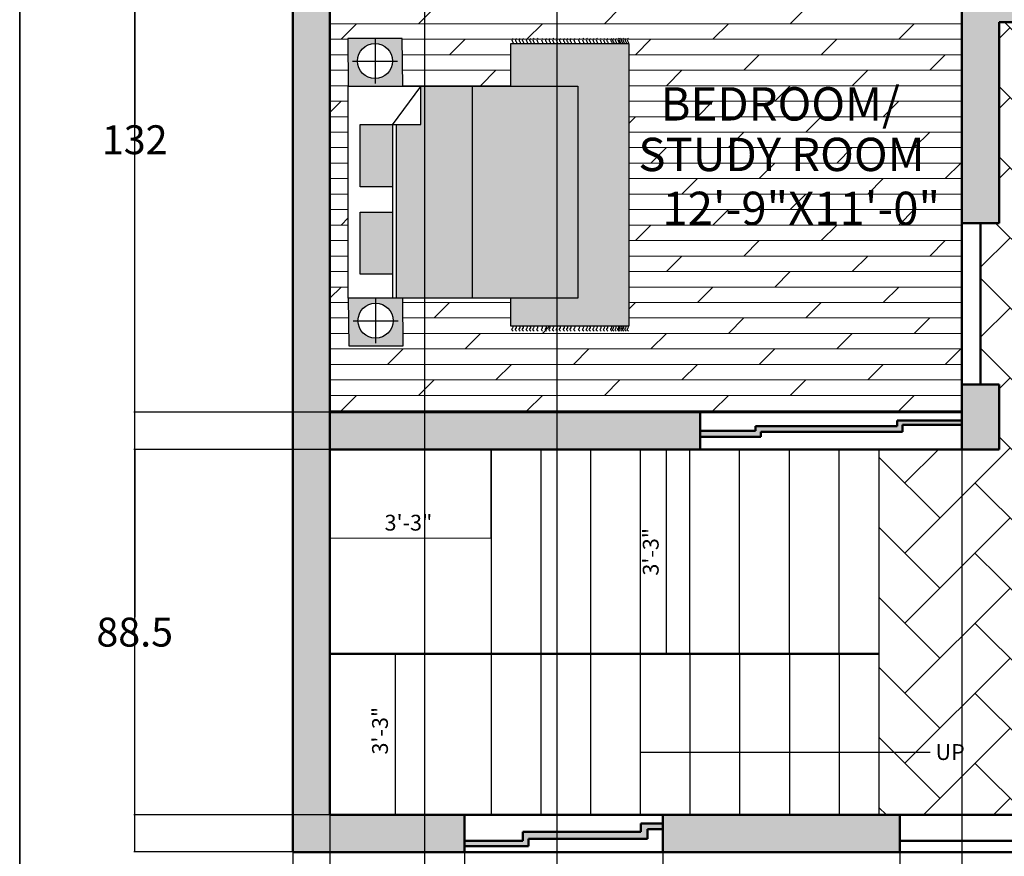
# Model space of a CAD drawing. Units: inches. Extents: x 1381 to 2246, y 1317 to 2168.
# Tile 2 of 15: x 1381 to 1619, y 1471 to 1673. Entities that reach past the tile are written whole.
import ezdxf

# ---------------------------------------------------------------- set-up
doc = ezdxf.new("R2010")
doc.units = ezdxf.units.IN
doc.header["$MEASUREMENT"] = 0
for name, color, linetype, lineweight in [('A-ANNO-DIMS', 2, 'Continuous', 18), ('A-ANNO-TEXT', 7, 'Continuous', 18), ('A-ANNO-TTLB', 7, 'Continuous', 35), ('A-AREA-IDEN', 3, 'Continuous', 25), ('A-FLOR-PATT', 252, 'Continuous', 13), ('A-FLOR-STRS', 3, 'Continuous', 25), ('A-FURN', 8, 'Continuous', 18), ('A-GLAZ', 4, 'Continuous', 25), ('A-WALL', 7, 'Continuous', 50)]:
    doc.layers.add(name, color=color, linetype=linetype, lineweight=lineweight)
doc.layers.add('furniture', color=250, linetype='Continuous')
doc.styles.get("Standard").update_dxf_attribs({"font": 'arial.ttf'})
doc.dimstyles.get("Standard").update_dxf_attribs({"dimtxt": 7, "dimasz": 0.18, "dimexe": 0.18, "dimexo": 0.0625, "dimgap": 0.09, "dimtad": 0, "dimtih": 1, "dimtoh": 1, "dimdec": 1, "dimzin": 0, "dimdsep": 46, "dimlunit": 3, "dimtxsty": 'Standard', "dimcen": 0.09, "dimadec": 0, "dimazin": 0, "dimtfac": 1, "dimtdec": 1, "dimtofl": 0, "dimtmove": 0, "dimatfit": 3, "dimfxl": 1, "dimtolj": 1, "dimtzin": 0, "dimarcsym": 0})

# ---------------------------------------------------------------- blocks, each defined once
blk = doc.blocks.new('CARPET')
at = {"layer": 'furniture'}
for p, q in [((-51.53, -98.11), (-51.53, -55.12)), ((-51.53, -55.12), (-41.27, -55.12)), ((36, -55.12), (51.55, -55.12)), ((51.55, -55.12), (51.55, -98.11)), ((51.55, -98.11), (-51.53, -98.11))]:
    blk.add_line(p, q, dxfattribs=at)
for points, knots in [([(-53.37, -55.99), (-53.22, -55.8), (-52.9, -55.41), (-52.34, -55.8), (-51.89, -56.08), (-51.65, -55.91), (-51.53, -55.83)], [0, 0, 0, 0, 0.653278, 1.290138, 1.740457, 2.114451, 2.114451, 2.114451, 2.114451]), ([(-53.37, -57.26), (-53.22, -57.07), (-52.9, -56.67), (-52.34, -57.07), (-51.89, -57.35), (-51.65, -57.17), (-51.53, -57.1)], [0, 0, 0, 0, 0.653278, 1.290138, 1.740457, 2.114451, 2.114451, 2.114451, 2.114451]), ([(53.37, -55.99), (53.22, -55.8), (52.9, -55.41), (52.34, -55.8), (51.89, -56.08), (51.65, -55.91), (51.53, -55.83)], [0, 0, 0, 0, 0.653278, 1.290138, 1.740457, 2.114451, 2.114451, 2.114451, 2.114451]), ([(53.37, -57.26), (53.22, -57.07), (52.9, -56.67), (52.34, -57.07), (51.89, -57.35), (51.65, -57.17), (51.53, -57.1)], [0, 0, 0, 0, 0.653278, 1.290138, 1.740457, 2.114451, 2.114451, 2.114451, 2.114451]), ([(-53.37, -58.59), (-53.22, -58.4), (-52.9, -58.01), (-52.34, -58.4), (-51.89, -58.68), (-51.65, -58.5), (-51.53, -58.43)], [0, 0, 0, 0, 0.653278, 1.290138, 1.740457, 2.114451, 2.114451, 2.114451, 2.114451]), ([(-53.37, -59.78), (-53.22, -59.58), (-52.9, -59.19), (-52.34, -59.58), (-51.89, -59.86), (-51.65, -59.69), (-51.53, -59.61)], [0, 0, 0, 0, 0.653278, 1.290138, 1.740457, 2.114451, 2.114451, 2.114451, 2.114451]), ([(-53.37, -61.22), (-53.22, -61.02), (-52.9, -60.63), (-52.34, -61.02), (-51.89, -61.3), (-51.65, -61.13), (-51.53, -61.05)], [0, 0, 0, 0, 0.653278, 1.290138, 1.740457, 2.114451, 2.114451, 2.114451, 2.114451]), ([(53.37, -58.59), (53.22, -58.4), (52.9, -58.01), (52.34, -58.4), (51.89, -58.68), (51.65, -58.5), (51.53, -58.43)], [0, 0, 0, 0, 0.653278, 1.290138, 1.740457, 2.114451, 2.114451, 2.114451, 2.114451]), ([(53.37, -59.78), (53.22, -59.58), (52.9, -59.19), (52.34, -59.58), (51.89, -59.86), (51.65, -59.69), (51.53, -59.61)], [0, 0, 0, 0, 0.653278, 1.290138, 1.740457, 2.114451, 2.114451, 2.114451, 2.114451]), ([(53.37, -61.22), (53.22, -61.02), (52.9, -60.63), (52.34, -61.02), (51.89, -61.3), (51.65, -61.13), (51.53, -61.05)], [0, 0, 0, 0, 0.653278, 1.290138, 1.740457, 2.114451, 2.114451, 2.114451, 2.114451]), ([(-53.37, -62.44), (-53.22, -62.25), (-52.9, -61.86), (-52.34, -62.25), (-51.89, -62.53), (-51.65, -62.36), (-51.53, -62.28)], [0, 0, 0, 0, 0.653278, 1.290138, 1.740457, 2.114451, 2.114451, 2.114451, 2.114451]), ([(-53.37, -63.63), (-53.22, -63.43), (-52.9, -63.04), (-52.34, -63.43), (-51.89, -63.72), (-51.65, -63.54), (-51.53, -63.46)], [0, 0, 0, 0, 0.653278, 1.290138, 1.740457, 2.114451, 2.114451, 2.114451, 2.114451]), ([(53.37, -62.44), (53.22, -62.25), (52.9, -61.86), (52.34, -62.25), (51.89, -62.53), (51.65, -62.36), (51.53, -62.28)], [0, 0, 0, 0, 0.653278, 1.290138, 1.740457, 2.114451, 2.114451, 2.114451, 2.114451]), ([(53.37, -63.63), (53.22, -63.43), (52.9, -63.04), (52.34, -63.43), (51.89, -63.72), (51.65, -63.54), (51.53, -63.46)], [0, 0, 0, 0, 0.653278, 1.290138, 1.740457, 2.114451, 2.114451, 2.114451, 2.114451]), ([(-53.37, -65.07), (-53.22, -64.87), (-52.9, -64.48), (-52.34, -64.87), (-51.89, -65.15), (-51.65, -64.98), (-51.53, -64.9)], [0, 0, 0, 0, 0.653278, 1.290138, 1.740457, 2.114451, 2.114451, 2.114451, 2.114451]), ([(-53.37, -66.76), (-53.22, -66.56), (-52.9, -66.17), (-52.34, -66.56), (-51.89, -66.84), (-51.65, -66.67), (-51.53, -66.59)], [0, 0, 0, 0, 0.653278, 1.290138, 1.740457, 2.114451, 2.114451, 2.114451, 2.114451]), ([(-53.37, -68.2), (-53.22, -68), (-52.9, -67.61), (-52.34, -68), (-51.89, -68.28), (-51.65, -68.11), (-51.53, -68.03)], [0, 0, 0, 0, 0.653278, 1.290138, 1.740457, 2.114451, 2.114451, 2.114451, 2.114451]), ([(53.37, -65.07), (53.22, -64.87), (52.9, -64.48), (52.34, -64.87), (51.89, -65.15), (51.65, -64.98), (51.53, -64.9)], [0, 0, 0, 0, 0.653278, 1.290138, 1.740457, 2.114451, 2.114451, 2.114451, 2.114451]), ([(53.37, -66.76), (53.22, -66.56), (52.9, -66.17), (52.34, -66.56), (51.89, -66.84), (51.65, -66.67), (51.53, -66.59)], [0, 0, 0, 0, 0.653278, 1.290138, 1.740457, 2.114451, 2.114451, 2.114451, 2.114451]), ([(53.37, -68.2), (53.22, -68), (52.9, -67.61), (52.34, -68), (51.89, -68.28), (51.65, -68.11), (51.53, -68.03)], [0, 0, 0, 0, 0.653278, 1.290138, 1.740457, 2.114451, 2.114451, 2.114451, 2.114451]), ([(-53.37, -69.53), (-53.22, -69.33), (-52.9, -68.94), (-52.34, -69.33), (-51.89, -69.61), (-51.65, -69.44), (-51.53, -69.36)], [0, 0, 0, 0, 0.653278, 1.290138, 1.740457, 2.114451, 2.114451, 2.114451, 2.114451]), ([(-53.37, -70.79), (-53.22, -70.6), (-52.9, -70.21), (-52.34, -70.6), (-51.89, -70.88), (-51.65, -70.7), (-51.53, -70.63)], [0, 0, 0, 0, 0.653278, 1.290138, 1.740457, 2.114451, 2.114451, 2.114451, 2.114451]), ([(-53.37, -72.12), (-53.22, -71.93), (-52.9, -71.54), (-52.34, -71.93), (-51.89, -72.21), (-51.65, -72.04), (-51.53, -71.96)], [0, 0, 0, 0, 0.653278, 1.290138, 1.740457, 2.114451, 2.114451, 2.114451, 2.114451]), ([(53.37, -69.53), (53.22, -69.33), (52.9, -68.94), (52.34, -69.33), (51.89, -69.61), (51.65, -69.44), (51.53, -69.36)], [0, 0, 0, 0, 0.653278, 1.290138, 1.740457, 2.114451, 2.114451, 2.114451, 2.114451]), ([(53.37, -70.79), (53.22, -70.6), (52.9, -70.21), (52.34, -70.6), (51.89, -70.88), (51.65, -70.7), (51.53, -70.63)], [0, 0, 0, 0, 0.653278, 1.290138, 1.740457, 2.114451, 2.114451, 2.114451, 2.114451]), ([(53.37, -72.12), (53.22, -71.93), (52.9, -71.54), (52.34, -71.93), (51.89, -72.21), (51.65, -72.04), (51.53, -71.96)], [0, 0, 0, 0, 0.653278, 1.290138, 1.740457, 2.114451, 2.114451, 2.114451, 2.114451]), ([(-53.37, -73.31), (-53.22, -73.11), (-52.9, -72.72), (-52.34, -73.11), (-51.89, -73.4), (-51.65, -73.22), (-51.53, -73.14)], [0, 0, 0, 0, 0.653278, 1.290138, 1.740457, 2.114451, 2.114451, 2.114451, 2.114451]), ([(-53.37, -74.75), (-53.22, -74.55), (-52.9, -74.16), (-52.34, -74.55), (-51.89, -74.83), (-51.65, -74.66), (-51.53, -74.58)], [0, 0, 0, 0, 0.653278, 1.290138, 1.740457, 2.114451, 2.114451, 2.114451, 2.114451]), ([(53.37, -73.31), (53.22, -73.11), (52.9, -72.72), (52.34, -73.11), (51.89, -73.4), (51.65, -73.22), (51.53, -73.14)], [0, 0, 0, 0, 0.653278, 1.290138, 1.740457, 2.114451, 2.114451, 2.114451, 2.114451]), ([(53.37, -74.75), (53.22, -74.55), (52.9, -74.16), (52.34, -74.55), (51.89, -74.83), (51.65, -74.66), (51.53, -74.58)], [0, 0, 0, 0, 0.653278, 1.290138, 1.740457, 2.114451, 2.114451, 2.114451, 2.114451]), ([(-53.37, -75.98), (-53.22, -75.78), (-52.9, -75.39), (-52.34, -75.78), (-51.89, -76.06), (-51.65, -75.89), (-51.53, -75.81)], [0, 0, 0, 0, 0.653278, 1.290138, 1.740457, 2.114451, 2.114451, 2.114451, 2.114451]), ([(-53.37, -77.16), (-53.22, -76.96), (-52.9, -76.57), (-52.34, -76.96), (-51.89, -77.25), (-51.65, -77.07), (-51.53, -76.99)], [0, 0, 0, 0, 0.653278, 1.290138, 1.740457, 2.114451, 2.114451, 2.114451, 2.114451]), ([(-53.37, -78.6), (-53.22, -78.4), (-52.9, -78.01), (-52.34, -78.4), (-51.89, -78.68), (-51.65, -78.51), (-51.53, -78.43)], [0, 0, 0, 0, 0.653278, 1.290138, 1.740457, 2.114451, 2.114451, 2.114451, 2.114451]), ([(53.37, -75.98), (53.22, -75.78), (52.9, -75.39), (52.34, -75.78), (51.89, -76.06), (51.65, -75.89), (51.53, -75.81)], [0, 0, 0, 0, 0.653278, 1.290138, 1.740457, 2.114451, 2.114451, 2.114451, 2.114451]), ([(53.37, -77.16), (53.22, -76.96), (52.9, -76.57), (52.34, -76.96), (51.89, -77.25), (51.65, -77.07), (51.53, -76.99)], [0, 0, 0, 0, 0.653278, 1.290138, 1.740457, 2.114451, 2.114451, 2.114451, 2.114451]), ([(53.37, -78.6), (53.22, -78.4), (52.9, -78.01), (52.34, -78.4), (51.89, -78.68), (51.65, -78.51), (51.53, -78.43)], [0, 0, 0, 0, 0.653278, 1.290138, 1.740457, 2.114451, 2.114451, 2.114451, 2.114451]), ([(-53.37, -80.29), (-53.22, -80.09), (-52.9, -79.7), (-52.34, -80.09), (-51.89, -80.37), (-51.65, -80.2), (-51.53, -80.12)], [0, 0, 0, 0, 0.653278, 1.290138, 1.740457, 2.114451, 2.114451, 2.114451, 2.114451]), ([(-53.37, -81.73), (-53.22, -81.53), (-52.9, -81.14), (-52.34, -81.53), (-51.89, -81.81), (-51.65, -81.64), (-51.53, -81.56)], [0, 0, 0, 0, 0.653278, 1.290138, 1.740457, 2.114451, 2.114451, 2.114451, 2.114451]), ([(53.37, -80.29), (53.22, -80.09), (52.9, -79.7), (52.34, -80.09), (51.89, -80.37), (51.65, -80.2), (51.53, -80.12)], [0, 0, 0, 0, 0.653278, 1.290138, 1.740457, 2.114451, 2.114451, 2.114451, 2.114451]), ([(53.37, -81.73), (53.22, -81.53), (52.9, -81.14), (52.34, -81.53), (51.89, -81.81), (51.65, -81.64), (51.53, -81.56)], [0, 0, 0, 0, 0.653278, 1.290138, 1.740457, 2.114451, 2.114451, 2.114451, 2.114451]), ([(-53.37, -83.06), (-53.22, -82.86), (-52.9, -82.47), (-52.34, -82.86), (-51.89, -83.14), (-51.65, -82.97), (-51.53, -82.89)], [0, 0, 0, 0, 0.653278, 1.290138, 1.740457, 2.114451, 2.114451, 2.114451, 2.114451]), ([(-53.37, -84.18), (-53.22, -83.99), (-52.9, -83.6), (-52.34, -83.99), (-51.89, -84.27), (-51.65, -84.09), (-51.53, -84.02)], [0, 0, 0, 0, 0.653278, 1.290138, 1.740457, 2.114451, 2.114451, 2.114451, 2.114451]), ([(-53.37, -85.51), (-53.22, -85.32), (-52.9, -84.93), (-52.34, -85.32), (-51.89, -85.6), (-51.65, -85.42), (-51.53, -85.35)], [0, 0, 0, 0, 0.653278, 1.290138, 1.740457, 2.114451, 2.114451, 2.114451, 2.114451]), ([(53.37, -83.06), (53.22, -82.86), (52.9, -82.47), (52.34, -82.86), (51.89, -83.14), (51.65, -82.97), (51.53, -82.89)], [0, 0, 0, 0, 0.653278, 1.290138, 1.740457, 2.114451, 2.114451, 2.114451, 2.114451]), ([(53.37, -84.18), (53.22, -83.99), (52.9, -83.6), (52.34, -83.99), (51.89, -84.27), (51.65, -84.09), (51.53, -84.02)], [0, 0, 0, 0, 0.653278, 1.290138, 1.740457, 2.114451, 2.114451, 2.114451, 2.114451]), ([(53.37, -85.51), (53.22, -85.32), (52.9, -84.93), (52.34, -85.32), (51.89, -85.6), (51.65, -85.42), (51.53, -85.35)], [0, 0, 0, 0, 0.653278, 1.290138, 1.740457, 2.114451, 2.114451, 2.114451, 2.114451]), ([(-53.37, -86.7), (-53.22, -86.5), (-52.9, -86.11), (-52.34, -86.5), (-51.89, -86.78), (-51.65, -86.61), (-51.53, -86.53)], [0, 0, 0, 0, 0.653278, 1.290138, 1.740457, 2.114451, 2.114451, 2.114451, 2.114451]), ([(-53.37, -88.14), (-53.22, -87.94), (-52.9, -87.55), (-52.34, -87.94), (-51.89, -88.22), (-51.65, -88.05), (-51.53, -87.97)], [0, 0, 0, 0, 0.653278, 1.290138, 1.740457, 2.114451, 2.114451, 2.114451, 2.114451]), ([(-53.37, -89.36), (-53.22, -89.17), (-52.9, -88.78), (-52.34, -89.17), (-51.89, -89.45), (-51.65, -89.28), (-51.53, -89.2)], [0, 0, 0, 0, 0.653278, 1.290138, 1.740457, 2.114451, 2.114451, 2.114451, 2.114451]), ([(53.37, -86.7), (53.22, -86.5), (52.9, -86.11), (52.34, -86.5), (51.89, -86.78), (51.65, -86.61), (51.53, -86.53)], [0, 0, 0, 0, 0.653278, 1.290138, 1.740457, 2.114451, 2.114451, 2.114451, 2.114451]), ([(53.37, -88.14), (53.22, -87.94), (52.9, -87.55), (52.34, -87.94), (51.89, -88.22), (51.65, -88.05), (51.53, -87.97)], [0, 0, 0, 0, 0.653278, 1.290138, 1.740457, 2.114451, 2.114451, 2.114451, 2.114451]), ([(53.37, -89.36), (53.22, -89.17), (52.9, -88.78), (52.34, -89.17), (51.89, -89.45), (51.65, -89.28), (51.53, -89.2)], [0, 0, 0, 0, 0.653278, 1.290138, 1.740457, 2.114451, 2.114451, 2.114451, 2.114451]), ([(-53.37, -90.55), (-53.22, -90.35), (-52.9, -89.96), (-52.34, -90.35), (-51.89, -90.64), (-51.65, -90.46), (-51.53, -90.38)], [0, 0, 0, 0, 0.653278, 1.290138, 1.740457, 2.114451, 2.114451, 2.114451, 2.114451]), ([(-53.37, -91.99), (-53.22, -91.79), (-52.9, -91.4), (-52.34, -91.79), (-51.89, -92.07), (-51.65, -91.9), (-51.53, -91.82)], [0, 0, 0, 0, 0.653278, 1.290138, 1.740457, 2.114451, 2.114451, 2.114451, 2.114451]), ([(-53.37, -92.69), (-53.22, -92.48), (-52.9, -92.08), (-52.35, -92.49), (-51.89, -92.77), (-51.65, -92.6), (-51.53, -92.52)], [0, 0, 0, 0, 0.663904, 1.307406, 1.757725, 2.131719, 2.131719, 2.131719, 2.131719]), ([(-53.37, -93.61), (-53.22, -93.42), (-52.9, -93.03), (-52.34, -93.42), (-51.89, -93.7), (-51.65, -93.52), (-51.53, -93.45)], [0, 0, 0, 0, 0.653278, 1.290138, 1.740457, 2.114451, 2.114451, 2.114451, 2.114451]), ([(53.37, -90.55), (53.22, -90.35), (52.9, -89.96), (52.34, -90.35), (51.9, -90.63), (51.66, -90.47), (51.55, -90.4)], [0, 0, 0, 0, 0.653278, 1.290138, 1.740457, 2.0926, 2.0926, 2.0926, 2.0926]), ([(53.37, -91.99), (53.22, -91.79), (52.9, -91.4), (52.34, -91.79), (51.9, -92.07), (51.66, -91.91), (51.55, -91.83)], [0, 0, 0, 0, 0.653278, 1.290138, 1.740457, 2.0926, 2.0926, 2.0926, 2.0926]), ([(53.37, -92.69), (53.22, -92.49), (52.9, -92.09), (52.34, -92.49), (51.9, -92.77), (51.66, -92.61), (51.55, -92.53)], [0, 0, 0, 0, 0.656792, 1.295826, 1.746145, 2.098292, 2.098292, 2.098292, 2.098292]), ([(53.37, -93.66), (53.22, -93.46), (52.9, -93.07), (52.34, -93.46), (51.9, -93.74), (51.66, -93.58), (51.55, -93.5)], [0, 0, 0, 0, 0.653278, 1.290138, 1.740457, 2.0926, 2.0926, 2.0926, 2.0926]), ([(-53.37, -94.55), (-53.22, -94.35), (-52.9, -93.96), (-52.34, -94.35), (-51.89, -94.63), (-51.65, -94.46), (-51.53, -94.38)], [0, 0, 0, 0, 0.653278, 1.290138, 1.740457, 2.114451, 2.114451, 2.114451, 2.114451]), ([(-53.37, -95.05), (-53.22, -94.85), (-52.9, -94.46), (-52.34, -94.85), (-51.89, -95.14), (-51.65, -94.96), (-51.53, -94.88)], [0, 0, 0, 0, 0.653278, 1.290138, 1.740457, 2.114451, 2.114451, 2.114451, 2.114451]), ([(-53.37, -95.73), (-53.22, -95.54), (-52.9, -95.15), (-52.34, -95.54), (-51.89, -95.82), (-51.65, -95.65), (-51.53, -95.57)], [0, 0, 0, 0, 0.653278, 1.290138, 1.740457, 2.114451, 2.114451, 2.114451, 2.114451]), ([(-53.37, -96.38), (-53.22, -96.18), (-52.9, -95.79), (-52.34, -96.18), (-51.89, -96.47), (-51.65, -96.29), (-51.53, -96.21)], [0, 0, 0, 0, 0.653278, 1.290138, 1.740457, 2.114451, 2.114451, 2.114451, 2.114451]), ([(-53.37, -97.17), (-53.22, -96.98), (-52.9, -96.59), (-52.34, -96.98), (-51.89, -97.26), (-51.65, -97.08), (-51.53, -97.01)], [0, 0, 0, 0, 0.653278, 1.290138, 1.740457, 2.114451, 2.114451, 2.114451, 2.114451]), ([(53.37, -95.78), (53.22, -95.58), (52.9, -95.19), (52.34, -95.58), (51.89, -95.86), (51.65, -95.69), (51.53, -95.61)], [0, 0, 0, 0, 0.653278, 1.290138, 1.740457, 2.114451, 2.114451, 2.114451, 2.114451]), ([(53.37, -96.43), (53.22, -96.23), (52.9, -95.84), (52.34, -96.23), (51.89, -96.51), (51.65, -96.34), (51.53, -96.26)], [0, 0, 0, 0, 0.653278, 1.290138, 1.740457, 2.114451, 2.114451, 2.114451, 2.114451]), ([(53.37, -97.22), (53.22, -97.02), (52.9, -96.63), (52.34, -97.02), (51.89, -97.3), (51.65, -97.13), (51.53, -97.05)], [0, 0, 0, 0, 0.653278, 1.290138, 1.740457, 2.114451, 2.114451, 2.114451, 2.114451]), ([(53.37, -94.59), (53.22, -94.4), (52.9, -94.01), (52.34, -94.4), (51.9, -94.68), (51.66, -94.51), (51.55, -94.44)], [0, 0, 0, 0, 0.653278, 1.290138, 1.740457, 2.0926, 2.0926, 2.0926, 2.0926]), ([(53.37, -95.1), (53.22, -94.9), (52.9, -94.51), (52.34, -94.9), (51.9, -95.18), (51.66, -95.02), (51.55, -94.94)], [0, 0, 0, 0, 0.653278, 1.290138, 1.740457, 2.0926, 2.0926, 2.0926, 2.0926]), ([(-53.37, -97.99), (-53.22, -97.79), (-52.9, -97.4), (-52.34, -97.79), (-51.89, -98.08), (-51.65, -97.9), (-51.53, -97.82)], [0, 0, 0, 0, 0.653278, 1.290138, 1.740457, 2.114451, 2.114451, 2.114451, 2.114451]), ([(53.37, -97.99), (53.22, -97.79), (52.9, -97.4), (52.34, -97.79), (51.89, -98.08), (51.65, -97.9), (51.53, -97.82)], [0, 0, 0, 0, 0.653278, 1.290138, 1.740457, 2.114451, 2.114451, 2.114451, 2.114451])]:
    blk.add_open_spline(points, degree=3, knots=knots, dxfattribs=at)
blk = doc.blocks.new('A$C58D270C6')
at = {"layer": 'furniture'}
for p, q in [((9.09, 124.13), (9.09, 108.87)), ((1.46, 116.5), (16.73, 116.5)), ((14.97, 94.84), (24.62, 107.92)), ((24.62, 94.93), (24.62, 107.92)), ((42.08, 108), (42.08, 36)), ((14.97, 94.93), (24.62, 94.93)), ((14.97, 94.84), (14.97, 36)), ((16.22, 94.93), (16.22, 36)), ((9.25, 36), (9.25, 20.74)), ((1.62, 28.37), (16.88, 28.37))]:
    blk.add_line(p, q, dxfattribs=at)
for points in [[(18.5, 108), (18.34, 124.13), (-0.16, 124.13), (0, 108)], [(0, 108), (77.91, 108), (77.91, 36), (0, 36)], [(4.09, 94.93), (14.97, 94.93), (14.97, 73.83), (4.09, 73.83)], [(4.09, 65.23), (14.97, 65.23), (14.97, 44.13), (4.09, 44.13)], [(18.65, 19.87), (18.5, 36), (0, 36), (0.16, 19.87)]]:
    blk.add_lwpolyline(points, close=True, dxfattribs=at)
for centre in [(9.09, 116.5), (9.25, 28.37)]:
    blk.add_circle(centre, 5.95, dxfattribs=at)
at = {"layer": 'furniture', "xscale": 0.9312884925094044, "yscale": 0.9312884925094044, "zscale": 0.9312884925094044, "rotation": 90}
blk.add_blockref('CARPET', (3.79, 74.47), dxfattribs=at)
blk = doc.blocks.new('*D49')
at = {"layer": 'A-ANNO-DIMS', "color": 0, "lineweight": -2, "transparency": 16777216}
for p, q in [((1447.05, 1471.85), (1447.05, 1384.36)), ((1746.55, 1471.85), (1746.55, 1384.36)), ((1447.23, 1384.54), (1584.81, 1384.54)), ((1746.37, 1384.54), (1608.79, 1384.54))]:
    blk.add_line(p, q, dxfattribs=at)
at = {"layer": 'A-ANNO-DIMS', "color": 0, "transparency": 16777216}
for points in [[(1447.23, 1384.57), (1447.23, 1384.51), (1447.05, 1384.54)], [(1746.37, 1384.57), (1746.37, 1384.51), (1746.55, 1384.54)]]:
    blk.add_solid(points, dxfattribs=at)
at = {"layer": 'Defpoints', "color": 0, "transparency": 16777216}
for p in [(1447.05, 1471.92), (1746.55, 1471.92), (1746.55, 1384.54)]:
    blk.add_point(p, dxfattribs=at)
at = {"layer": 'A-ANNO-DIMS', "color": 0, "transparency": 16777216, "insert": (1596.8, 1384.54), "char_height": 7, "attachment_point": 5}
blk.add_mtext('\\A1;299.5', dxfattribs=at)
blk = doc.blocks.new('*D50')
at = {"layer": 'A-ANNO-DIMS', "color": 0, "lineweight": -2, "transparency": 16777216}
for p, q in [((1446.99, 2092.92), (1408.62, 2092.92)), ((1408.8, 2092.74), (1408.8, 1786.08)), ((1408.8, 1472.1), (1408.8, 1778.75)), ((1446.99, 1471.92), (1408.62, 1471.92))]:
    blk.add_line(p, q, dxfattribs=at)
at = {"layer": 'A-ANNO-DIMS', "color": 0, "transparency": 16777216}
for points in [[(1408.77, 2092.74), (1408.83, 2092.74), (1408.8, 2092.92)], [(1408.77, 1472.1), (1408.83, 1472.1), (1408.8, 1471.92)]]:
    blk.add_solid(points, dxfattribs=at)
at = {"layer": 'Defpoints', "color": 0, "transparency": 16777216}
for p in [(1408.8, 2092.92), (1447.05, 2092.92), (1447.05, 1471.92)]:
    blk.add_point(p, dxfattribs=at)
at = {"layer": 'A-ANNO-DIMS', "color": 0, "transparency": 16777216, "insert": (1408.8, 1782.42), "char_height": 7, "attachment_point": 5}
blk.add_mtext('\\A1;621', dxfattribs=at)
blk = doc.blocks.new('*D54')
at = {"layer": 'A-ANNO-DIMS', "color": 0, "lineweight": -2, "transparency": 16777216}
for p, q in [((1455.99, 1569.42), (1408.62, 1569.42)), ((1408.8, 1569.24), (1408.8, 1528.83)), ((1408.8, 1481.1), (1408.8, 1521.5)), ((1455.99, 1480.92), (1408.62, 1480.92))]:
    blk.add_line(p, q, dxfattribs=at)
at = {"layer": 'A-ANNO-DIMS', "color": 0, "transparency": 16777216}
for points in [[(1408.77, 1569.24), (1408.83, 1569.24), (1408.8, 1569.42)], [(1408.77, 1481.1), (1408.83, 1481.1), (1408.8, 1480.92)]]:
    blk.add_solid(points, dxfattribs=at)
at = {"layer": 'Defpoints', "color": 0, "transparency": 16777216}
for p in [(1408.8, 1569.42), (1456.05, 1569.42), (1456.05, 1480.92)]:
    blk.add_point(p, dxfattribs=at)
at = {"layer": 'A-ANNO-DIMS', "color": 0, "transparency": 16777216, "insert": (1408.8, 1525.17), "char_height": 7, "attachment_point": 5}
blk.add_mtext('\\A1;88.5', dxfattribs=at)
blk = doc.blocks.new('*D55')
at = {"layer": 'A-ANNO-DIMS', "color": 0, "lineweight": -2, "transparency": 16777216}
for p, q in [((1455.99, 1710.42), (1408.62, 1710.42)), ((1408.8, 1710.24), (1408.8, 1648.08)), ((1408.8, 1578.6), (1408.8, 1640.75)), ((1455.99, 1578.42), (1408.62, 1578.42))]:
    blk.add_line(p, q, dxfattribs=at)
at = {"layer": 'A-ANNO-DIMS', "color": 0, "transparency": 16777216}
for points in [[(1408.77, 1710.24), (1408.83, 1710.24), (1408.8, 1710.42)], [(1408.77, 1578.6), (1408.83, 1578.6), (1408.8, 1578.42)]]:
    blk.add_solid(points, dxfattribs=at)
at = {"layer": 'Defpoints', "color": 0, "transparency": 16777216}
for p in [(1408.8, 1710.42), (1456.05, 1710.42), (1456.05, 1578.42)]:
    blk.add_point(p, dxfattribs=at)
at = {"layer": 'A-ANNO-DIMS', "color": 0, "transparency": 16777216, "insert": (1408.8, 1644.42), "char_height": 7, "attachment_point": 5}
blk.add_mtext('\\A1;132', dxfattribs=at)
blk = doc.blocks.new('*D62')
at = {"layer": 'A-ANNO-DIMS', "color": 0, "lineweight": -2, "transparency": 16777216}
for p, q in [((1447.05, 1471.85), (1447.05, 1384.36)), ((1488.66, 1471.85), (1488.66, 1384.36)), ((1447.23, 1384.54), (1456.49, 1384.54)), ((1488.48, 1384.54), (1479.22, 1384.54))]:
    blk.add_line(p, q, dxfattribs=at)
at = {"layer": 'A-ANNO-DIMS', "color": 0, "transparency": 16777216}
for points in [[(1447.23, 1384.57), (1447.23, 1384.51), (1447.05, 1384.54)], [(1488.48, 1384.57), (1488.48, 1384.51), (1488.66, 1384.54)]]:
    blk.add_solid(points, dxfattribs=at)
at = {"layer": 'Defpoints', "color": 0, "transparency": 16777216}
for p in [(1447.05, 1471.92), (1488.66, 1471.92), (1488.66, 1384.54)]:
    blk.add_point(p, dxfattribs=at)
at = {"layer": 'A-ANNO-DIMS', "color": 0, "transparency": 16777216, "insert": (1467.86, 1384.54), "char_height": 7, "attachment_point": 5}
blk.add_mtext('\\A1;41.61', dxfattribs=at)
blk = doc.blocks.new('*D63')
at = {"layer": 'A-ANNO-DIMS', "color": 0, "lineweight": -2, "transparency": 16777216}
for p, q in [((1488.66, 1471.85), (1488.66, 1384.36)), ((1536.65, 1471.85), (1536.65, 1384.36)), ((1488.84, 1384.54), (1500.61, 1384.54)), ((1536.47, 1384.54), (1524.7, 1384.54))]:
    blk.add_line(p, q, dxfattribs=at)
at = {"layer": 'A-ANNO-DIMS', "color": 0, "transparency": 16777216}
for points in [[(1488.84, 1384.57), (1488.84, 1384.51), (1488.66, 1384.54)], [(1536.47, 1384.57), (1536.47, 1384.51), (1536.65, 1384.54)]]:
    blk.add_solid(points, dxfattribs=at)
at = {"layer": 'Defpoints', "color": 0, "transparency": 16777216}
for p in [(1488.66, 1471.92), (1536.65, 1471.92), (1536.65, 1384.54)]:
    blk.add_point(p, dxfattribs=at)
at = {"layer": 'A-ANNO-DIMS', "color": 0, "transparency": 16777216, "insert": (1512.65, 1384.54), "char_height": 7, "attachment_point": 5}
blk.add_mtext('\\A1;47.98', dxfattribs=at)
blk = doc.blocks.new('*D64')
at = {"layer": 'A-ANNO-DIMS', "color": 0, "lineweight": -2, "transparency": 16777216}
for p, q in [((1536.65, 1471.85), (1536.65, 1384.36)), ((1594.05, 1471.85), (1594.05, 1384.36)), ((1536.83, 1384.54), (1556.18, 1384.54)), ((1593.87, 1384.54), (1574.51, 1384.54))]:
    blk.add_line(p, q, dxfattribs=at)
at = {"layer": 'A-ANNO-DIMS', "color": 0, "transparency": 16777216}
for points in [[(1536.83, 1384.57), (1536.83, 1384.51), (1536.65, 1384.54)], [(1593.87, 1384.57), (1593.87, 1384.51), (1594.05, 1384.54)]]:
    blk.add_solid(points, dxfattribs=at)
at = {"layer": 'Defpoints', "color": 0, "transparency": 16777216}
for p in [(1536.65, 1471.92), (1594.05, 1471.92), (1594.05, 1384.54)]:
    blk.add_point(p, dxfattribs=at)
at = {"layer": 'A-ANNO-DIMS', "color": 0, "transparency": 16777216, "insert": (1565.35, 1384.54), "char_height": 7, "attachment_point": 5}
blk.add_mtext('\\A1;57.4', dxfattribs=at)
blk = doc.blocks.new('*D65')
at = {"layer": 'A-ANNO-DIMS', "color": 0, "lineweight": -2, "transparency": 16777216}
for p, q in [((1594.05, 1471.85), (1594.05, 1384.36)), ((1726.05, 1471.85), (1726.05, 1384.36)), ((1594.23, 1384.54), (1652.59, 1384.54)), ((1725.87, 1384.54), (1667.5, 1384.54))]:
    blk.add_line(p, q, dxfattribs=at)
at = {"layer": 'A-ANNO-DIMS', "color": 0, "transparency": 16777216}
for points in [[(1594.23, 1384.57), (1594.23, 1384.51), (1594.05, 1384.54)], [(1725.87, 1384.57), (1725.87, 1384.51), (1726.05, 1384.54)]]:
    blk.add_solid(points, dxfattribs=at)
at = {"layer": 'Defpoints', "color": 0, "transparency": 16777216}
for p in [(1594.05, 1471.92), (1726.05, 1471.92), (1726.05, 1384.54)]:
    blk.add_point(p, dxfattribs=at)
at = {"layer": 'A-ANNO-DIMS', "color": 0, "transparency": 16777216, "insert": (1660.05, 1384.54), "char_height": 7, "attachment_point": 5}
blk.add_mtext('\\A1;132', dxfattribs=at)
blk = doc.blocks.new('*D66')
at = {"layer": 'A-ANNO-DIMS', "color": 0, "lineweight": -2, "transparency": 16777216}
for p, q in [((1456.05, 1578.35), (1456.05, 1384.36)), ((1609.05, 1578.35), (1609.05, 1384.36)), ((1456.23, 1384.54), (1525.06, 1384.54)), ((1608.87, 1384.54), (1540.04, 1384.54))]:
    blk.add_line(p, q, dxfattribs=at)
at = {"layer": 'A-ANNO-DIMS', "color": 0, "transparency": 16777216}
for points in [[(1456.23, 1384.57), (1456.23, 1384.51), (1456.05, 1384.54)], [(1608.87, 1384.57), (1608.87, 1384.51), (1609.05, 1384.54)]]:
    blk.add_solid(points, dxfattribs=at)
at = {"layer": 'Defpoints', "color": 0, "transparency": 16777216}
for p in [(1456.05, 1578.42), (1609.05, 1578.42), (1609.05, 1384.54)]:
    blk.add_point(p, dxfattribs=at)
at = {"layer": 'A-ANNO-DIMS', "color": 0, "transparency": 16777216, "insert": (1532.55, 1384.54), "char_height": 7, "attachment_point": 5}
blk.add_mtext('\\A1;153', dxfattribs=at)
blk = doc.blocks.new('*D67')
at = {"layer": 'A-ANNO-DIMS', "color": 0, "lineweight": -2, "transparency": 16777216}
for p, q in [((1456.050973, 1911.353813), (1456.050973, 1384.360695)), ((1478.962127, 1911.353813), (1478.962127, 1384.360695)), ((1455.870973, 1384.540695), (1455.690973, 1384.540695)), ((1479.142127, 1384.540695), (1479.322127, 1384.540695))]:
    blk.add_line(p, q, dxfattribs=at)
at = {"layer": 'A-ANNO-DIMS', "color": 0, "transparency": 16777216}
for points in [[(1455.870973, 1384.570695), (1455.870973, 1384.510695), (1456.050973, 1384.540695)], [(1479.142127, 1384.570695), (1479.142127, 1384.510695), (1478.962127, 1384.540695)]]:
    blk.add_solid(points, dxfattribs=at)
at = {"layer": 'Defpoints', "color": 0, "transparency": 16777216}
for p in [(1456.050973, 1911.416313), (1478.962127, 1911.416313), (1478.962127, 1384.540695)]:
    blk.add_point(p, dxfattribs=at)
at = {"layer": 'A-ANNO-DIMS', "color": 0, "transparency": 16777216, "insert": (1467.50655, 1384.540695), "char_height": 7, "attachment_point": 5}
blk.add_mtext('\\A1;22.91', dxfattribs=at)
blk = doc.blocks.new('*D68')
at = {"layer": 'A-ANNO-DIMS', "color": 0, "lineweight": -2, "transparency": 16777216}
for p, q in [((1478.96, 1911.35), (1478.96, 1384.36)), ((1511.02, 1911.35), (1511.02, 1384.36)), ((1479.14, 1384.54), (1480.39, 1384.54)), ((1510.84, 1384.54), (1509.59, 1384.54))]:
    blk.add_line(p, q, dxfattribs=at)
at = {"layer": 'A-ANNO-DIMS', "color": 0, "transparency": 16777216}
for points in [[(1479.14, 1384.57), (1479.14, 1384.51), (1478.96, 1384.54)], [(1510.84, 1384.57), (1510.84, 1384.51), (1511.02, 1384.54)]]:
    blk.add_solid(points, dxfattribs=at)
at = {"layer": 'Defpoints', "color": 0, "transparency": 16777216}
for p in [(1478.96, 1911.42), (1511.02, 1911.42), (1511.02, 1384.54)]:
    blk.add_point(p, dxfattribs=at)
at = {"layer": 'A-ANNO-DIMS', "color": 0, "transparency": 16777216, "insert": (1494.99, 1384.54), "char_height": 7, "attachment_point": 5}
blk.add_mtext('\\A1;32.054', dxfattribs=at)

msp = doc.modelspace()

# ---------------------------------------------------------------- hatches: boundary and pattern name
at = {"layer": 'A-FLOR-PATT'}
h = msp.add_hatch(dxfattribs=at)
h.set_pattern_fill('DOLMIT', color=256, scale=15)
h.paths.add_polyline_path([(1609.051, 1710.4163), (1517.1194, 1710.4163), (1517.1194, 1683.9148), (1456.051, 1683.9148), (1456.051, 1578.4163), (1545.7088, 1578.4163), (1609.051, 1578.4163)])
h.paths.add_polyline_path([(1528.374, 1667.7293), (1528.374, 1599.2474), (1499.8186, 1599.2474), (1499.8186, 1606.0382), (1473.6909, 1606.0382), (1473.8019, 1594.5315), (1460.606, 1594.5315), (1460.4951, 1606.0382), (1460.4951, 1657.3975), (1460.3841, 1668.9042), (1473.5799, 1668.9042), (1473.6909, 1657.3975), (1499.8186, 1657.3975), (1499.8186, 1667.7293)], flags=16)
h.paths.add_polyline_path([(1478.0548, 1657.3422), (1478.0548, 1648.0757), (1471.2225, 1648.0757), (1471.1765, 1648.0133), (1471.1765, 1611.8376), (1463.4157, 1611.8376), (1463.4157, 1626.8866), (1471.1765, 1626.8866), (1471.1765, 1633.0267), (1463.4157, 1633.0267), (1463.4157, 1648.0757), (1471.2225, 1648.0757)], flags=0)
h.paths.add_polyline_path([(1471.2297, 1663.4608, -1), (1462.7343, 1663.4608, -1)], flags=0)
h.paths.add_polyline_path([(1471.3407, 1600.5947, -1), (1462.8453, 1600.5947, -1)], flags=0)
h.paths.add_polyline_path([(1534.4824, 1621.5603), (1603.5976, 1621.5603), (1603.5976, 1633.9282), (1534.4824, 1633.9282)], flags=24)
h.paths.add_polyline_path([(1528.6332, 1634.5998), (1609.2654, 1634.5998), (1609.2654, 1647.1329), (1528.6332, 1647.1329)], flags=9)
h.paths.add_polyline_path([(1534.0271, 1646.8395), (1599.6229, 1646.8395), (1599.6229, 1659.3726), (1534.0271, 1659.3726)], flags=24)
h = msp.add_hatch(dxfattribs=at)
h.set_pattern_fill('AR-HBONE', color=256, scale=3)
h.paths.add_polyline_path([(1737.551, 1672.9163), (1732.8596, 1672.9163), (1699.1735, 1672.9163), (1618.051, 1672.9163), (1618.051, 1624.2465), (1613.551, 1624.2465), (1613.551, 1585.1257), (1618.051, 1585.1257), (1618.051, 1569.4163), (1609.051, 1569.4163), (1588.9723, 1569.4163), (1588.9723, 1480.9163), (1594.0453, 1480.9163), (1726.0453, 1480.9163), (1726.0453, 1471.9163), (1737.551, 1471.9163)])
at = {"layer": 'A-FURN'}
h = msp.add_hatch(color=256, dxfattribs=at)
h.dxf.hatch_style = 1
h.paths.add_polyline_path([(1528.374, 1667.7293), (1499.8186, 1667.7293), (1499.8186, 1657.3975), (1516.0666, 1657.3975), (1516.0666, 1606.0382), (1499.8186, 1606.0382), (1499.8186, 1599.2474), (1528.374, 1599.2474)])
h.paths.add_polyline_path([(1467.093, 1606.0382), (1460.4951, 1606.0382), (1460.606, 1594.5315), (1473.8019, 1594.5315), (1473.6909, 1606.0382), (1467.093, 1606.0382), (1467.093, 1604.8424, -0.41421356), (1471.3407, 1600.5947, -1), (1462.8453, 1600.5947, -0.41421356), (1467.093, 1604.8424)])
h.paths.add_polyline_path([(1473.5799, 1668.9042), (1466.982, 1668.9042), (1466.982, 1667.7085, -0.41421356), (1471.2297, 1663.4608, -1), (1462.7343, 1663.4608, -0.41421356), (1466.982, 1667.7085), (1466.982, 1668.9042), (1460.3841, 1668.9042), (1460.4951, 1657.3975), (1473.6909, 1657.3975)])
h = msp.add_hatch(color=256, dxfattribs=at)
h.dxf.hatch_style = 1
h.paths.add_polyline_path([(1490.5104, 1657.3975), (1478.0956, 1657.3975), (1478.0548, 1657.3422), (1478.0548, 1648.0757), (1472.0629, 1648.0757), (1472.0629, 1606.0382), (1490.5104, 1606.0382)])
h.paths.add_polyline_path([(1516.0666, 1657.3975), (1490.5104, 1657.3975), (1490.5104, 1606.0382), (1516.0666, 1606.0382)])
h = msp.add_hatch(color=256, dxfattribs=at)
h.dxf.hatch_style = 1
h.paths.add_polyline_path([(1471.1765, 1626.8866), (1463.4157, 1626.8866), (1463.4157, 1611.8376), (1471.1765, 1611.8376)])
h.paths.add_polyline_path([(1471.1765, 1648.0757), (1463.4157, 1648.0757), (1463.4157, 1633.0267), (1471.1765, 1633.0267)])
at = {"layer": 'A-GLAZ'}
h = msp.add_hatch(color=256, dxfattribs=at)
h.dxf.hatch_style = 1
h.paths.add_polyline_path([(1456.051, 2083.9163), (1737.551, 2083.9163), (1737.551, 1677.4163), (1732.8596, 1677.4163), (1732.8596, 1672.9163), (1737.551, 1672.9163), (1737.551, 1471.9163), (1746.551, 1471.9163), (1746.551, 2092.9163), (1447.051, 2092.9163), (1447.051, 2083.9163), (1447.051, 1471.9163), (1488.6632, 1471.9163), (1488.6632, 1480.9163), (1456.051, 1480.9163), (1456.051, 1710.4163), (1517.1194, 1710.4163), (1517.1194, 1714.9163), (1491.551, 1714.9163), (1491.551, 1729.193), (1487.051, 1729.193), (1487.051, 1714.9163), (1456.051, 1714.9163)])
h.paths.add_polyline_path([(1622.551, 2035.4163), (1625.0954, 2035.4163), (1625.0954, 2039.9163), (1618.051, 2039.9163), (1618.051, 1915.9163), (1611.2353, 1915.9163), (1611.2353, 1911.4163), (1626.5102, 1911.4163), (1626.5102, 1915.9163), (1622.551, 1915.9163)], flags=17)
h.paths.add_polyline_path([(1737.551, 1915.9163), (1668.5102, 1915.9163), (1668.5102, 1911.4163), (1737.551, 1911.4163)], flags=17)
h.paths.add_polyline_path([(1682.2831, 2039.9163), (1655.8191, 2039.9163), (1655.8191, 2035.4163), (1682.2831, 2035.4163)], flags=17)
h.paths.add_polyline_path([(1737.551, 2039.9163), (1725.9636, 2039.9163), (1725.9636, 2035.4163), (1737.551, 2035.4163)], flags=17)
h.paths.add_polyline_path([(1684.2508, 1711.4667), (1740.8192, 1711.4667), (1740.8192, 1723.8346), (1684.2508, 1723.8346)], flags=25)
h = msp.add_hatch(color=256, dxfattribs=at)
h.dxf.hatch_style = 1
h.paths.add_polyline_path([(1478.9621, 1915.9163), (1456.051, 1915.9163), (1456.051, 1911.4163), (1478.9621, 1911.4163)])
h.paths.add_polyline_path([(1566.2107, 1915.9163), (1511.016, 1915.9163), (1511.016, 1911.4163), (1516.051, 1911.4163), (1516.051, 1779.4163), (1484.0852, 1779.4163), (1484.0852, 1774.9163), (1487.051, 1774.9163), (1487.051, 1755.1129), (1491.551, 1755.1129), (1491.551, 1774.9163), (1563.551, 1774.9163), (1563.551, 1770.3401), (1568.051, 1770.3401), (1568.051, 1779.4163), (1520.551, 1779.4163), (1520.551, 1911.4163), (1566.2107, 1911.4163)])
h.paths.add_polyline_path([(1568.051, 1734.7997), (1563.551, 1734.7997), (1563.551, 1714.9163), (1557.5961, 1714.9163), (1557.5961, 1710.4163), (1568.051, 1710.4163)])
h.paths.add_polyline_path([(1458.1653, 1779.4163), (1456.051, 1779.4163), (1456.051, 1774.9163), (1458.1653, 1774.9163)])
h.paths.add_polyline_path([(1684.551, 1746.8536), (1680.051, 1746.8536), (1680.051, 1677.4163), (1673.5117, 1677.4163), (1673.5117, 1672.9163), (1699.1735, 1672.9163), (1699.1735, 1677.4163), (1684.551, 1677.4163)])
h.paths.add_polyline_path([(1613.551, 1746.8536), (1609.051, 1746.8536), (1609.051, 1624.2465), (1618.051, 1624.2465), (1618.051, 1672.9163), (1625.5117, 1672.9163), (1625.5117, 1677.4163), (1613.551, 1677.4163)])
h.paths.add_polyline_path([(1618.051, 1585.1257), (1609.051, 1585.1257), (1609.051, 1569.4163), (1618.051, 1569.4163)])
h.paths.add_polyline_path([(1545.7088, 1578.4163), (1456.051, 1578.4163), (1456.051, 1569.4163), (1545.7088, 1569.4163)])
h.paths.add_polyline_path([(1594.0453, 1480.9163), (1536.6467, 1480.9163), (1536.6467, 1471.9163), (1594.0453, 1471.9163)])
h = msp.add_hatch(color=256, dxfattribs=at)
h.dxf.hatch_style = 1
h.paths.add_polyline_path([(1560.3463, 1573.662), (1594.6347, 1573.662), (1594.6347, 1575.3695), (1609.051, 1575.3695), (1609.051, 1576.4366), (1593.3529, 1576.4366), (1593.3529, 1575.0493), (1559.0645, 1575.0493), (1559.0645, 1573.9163), (1545.7088, 1573.9163), (1545.7088, 1572.4881), (1560.3463, 1572.4881)])
h = msp.add_hatch(color=256, dxfattribs=at)
h.dxf.hatch_style = 1
h.paths.add_polyline_path([(1504.1205, 1475.1168), (1532.9106, 1475.1168), (1532.9106, 1477.4669), (1536.6467, 1477.4669), (1536.6467, 1478.8247), (1531.2989, 1478.8247), (1531.2989, 1476.8141), (1502.7286, 1476.8141), (1502.7286, 1474.6468), (1488.6632, 1474.6468), (1488.6632, 1473.3412), (1504.1205, 1473.3412)])

# ---------------------------------------------------------------- linework, layer by layer
at = {"layer": 'A-ANNO-DIMS'}
msp.add_line((1456.051, 1547.9259), (1495.051, 1547.9259), dxfattribs=at)
at = {"layer": 'A-ANNO-TTLB'}
msp.add_line((1380.9518, 1316.7761), (1380.9518, 2167.8236), dxfattribs=at)
at = {"layer": 'A-FLOR-STRS'}
for p, q in [((1495.051, 1547.9259), (1495.051, 1569.4163)), ((1495.051, 1569.4163), (1495.051, 1480.9163)), ((1507.0885, 1569.4163), (1507.0885, 1480.9163)), ((1519.1259, 1569.4163), (1519.1259, 1480.9163)), ((1531.1634, 1569.4163), (1531.1634, 1480.9163)), ((1537.4908, 1569.4163), (1537.4908, 1519.9163)), ((1543.2009, 1519.9163), (1543.2009, 1569.4163)), ((1555.2384, 1519.9163), (1555.2384, 1569.4163)), ((1567.2759, 1519.9163), (1567.2759, 1569.4163)), ((1579.3134, 1519.9163), (1579.3134, 1569.4163)), ((1588.9723, 1569.4163), (1588.9723, 1480.9163)), ((1471.9159, 1480.9163), (1471.9159, 1519.9163)), ((1543.2009, 1519.9163), (1543.2009, 1480.9163)), ((1555.2384, 1519.9163), (1555.2384, 1480.9163)), ((1567.2759, 1519.9163), (1567.2759, 1480.9163)), ((1579.3134, 1519.9163), (1579.3134, 1480.9163)), ((1531.1634, 1496.1305), (1585.3427, 1496.1305)), ((1585.3427, 1496.1305), (1601.4017, 1496.1305)), ((1536.6467, 1480.9163), (1488.6632, 1480.9163))]:
    msp.add_line(p, q, dxfattribs=at)
at = {"layer": 'A-WALL'}
for p, q in [((1447.051, 2083.9163), (1447.051, 1471.9163)), ((1609.051, 1746.8536), (1609.051, 1569.4163)), ((1456.051, 1710.4163), (1456.051, 1480.9163)), ((1618.051, 1672.9163), (1618.051, 1624.2465)), ((1618.051, 1672.9163), (1699.1735, 1672.9163)), ((1609.051, 1624.2465), (1618.051, 1624.2465)), ((1613.551, 1585.1257), (1613.551, 1624.2465)), ((1609.051, 1585.1257), (1618.051, 1585.1257)), ((1618.051, 1585.1257), (1618.051, 1569.4163)), ((1456.051, 1578.4163), (1545.7088, 1578.4163)), ((1545.7088, 1578.4163), (1545.7088, 1569.4163)), ((1545.7088, 1578.4163), (1609.051, 1578.4163)), ((1609.051, 1569.4163), (1609.051, 1578.4163)), ((1593.3529, 1575.0493), (1593.3529, 1576.4366)), ((1593.3529, 1576.4366), (1609.051, 1576.4366)), ((1545.7088, 1573.9163), (1559.0645, 1573.9163)), ((1559.0645, 1573.9163), (1559.0645, 1575.0493)), ((1559.0645, 1575.0493), (1593.3529, 1575.0493)), ((1560.3463, 1572.4881), (1560.3463, 1573.662)), ((1560.3463, 1573.662), (1594.6347, 1573.662)), ((1594.6347, 1573.662), (1594.6347, 1575.3695)), ((1594.6347, 1575.3695), (1609.051, 1575.3695)), ((1545.7088, 1572.4881), (1560.3463, 1572.4881)), ((1456.051, 1569.4163), (1545.7088, 1569.4163)), ((1545.7088, 1569.4163), (1609.051, 1569.4163)), ((1609.051, 1569.4163), (1618.051, 1569.4163)), ((1471.9159, 1519.9163), (1456.051, 1519.9163)), ((1456.051, 1519.9163), (1588.9723, 1519.9163)), ((1456.051, 1480.9163), (1594.0453, 1480.9163)), ((1488.6632, 1480.9163), (1488.6632, 1471.9163)), ((1488.6632, 1480.9163), (1488.6632, 1474.6468)), ((1536.6467, 1471.9163), (1536.6467, 1480.9163)), ((1594.0453, 1480.9163), (1594.0453, 1471.9163)), ((1594.0453, 1480.9163), (1726.0453, 1480.9163)), ((1531.2989, 1476.8141), (1531.2989, 1478.8247)), ((1531.2989, 1478.8247), (1536.6467, 1478.8247)), ((1502.7286, 1474.6468), (1502.7286, 1476.8141)), ((1502.7286, 1476.8141), (1531.2989, 1476.8141)), ((1532.9106, 1475.1168), (1532.9106, 1477.4669)), ((1532.9106, 1477.4669), (1536.6467, 1477.4669)), ((1488.6632, 1474.6468), (1502.7286, 1474.6468)), ((1488.6632, 1473.3412), (1504.1205, 1473.3412)), ((1504.1205, 1473.3412), (1504.1205, 1475.1168)), ((1504.1205, 1475.1168), (1532.9106, 1475.1168)), ((1594.0453, 1474.6181), (1726.0453, 1474.6181)), ((1447.051, 1471.9163), (1746.551, 1471.9163)), ((1488.6632, 1471.9163), (1536.6467, 1471.9163))]:
    msp.add_line(p, q, dxfattribs=at)

# ---------------------------------------------------------------- block references
at = {"layer": 'A-FURN', "xscale": 0.7133243416521088, "yscale": 0.7133243416521088, "zscale": 0.7133243416521088}
msp.add_blockref('A$C58D270C6', (1460.4951, 1580.3585), dxfattribs=at)

# ---------------------------------------------------------------- texts
at = {"layer": 'A-ANNO-TEXT'}
for s, p in [('3\'-3"', (1469.2783, 1549.7601)), ('UP', (1602.6558, 1494.2051))]:
    msp.add_text(s, height=3.83139, dxfattribs=at).set_placement(p)
for p in [(1535.6289, 1538.8518), (1470.0929, 1495.5207)]:
    msp.add_text('3\'-3"', height=3.83139, rotation=90, dxfattribs=at).set_placement(p)
at = {"layer": 'A-AREA-IDEN'}
for s, height, p in [('BEDROOM/', 8.07451, (1536.116, 1649.066)), ('STUDY ROOM', 8.07451, (1530.722, 1636.8264)), ('12\'-9"X11\'-0"', 8.074511, (1536.5437, 1623.7593))]:
    msp.add_text(s, height=height, dxfattribs=at).set_placement(p)

# ---------------------------------------------------------------- dimensions: what is measured, and where the dimension line sits
at = {"layer": 'A-ANNO-DIMS'}
for base, p1, p2, override, picture, middle in [((1408.801, 2092.9163), (1447.051, 1471.9163), (1447.051, 2092.9163), {"dimdec": 0, "dimlfac": 1, "dimrnd": 0, "dimzin": 0, "dimdsep": 46, "dimlunit": 2}, '*D50', (1408.801, 1782.4163)), ((1408.801, 1710.4163), (1456.051, 1578.4163), (1456.051, 1710.4163), {"dimdec": 0, "dimlfac": 1, "dimrnd": 0, "dimzin": 0, "dimdsep": 46, "dimlunit": 2}, '*D55', (1408.801, 1644.4163)), ((1408.801, 1569.4163), (1456.051, 1480.9163), (1456.051, 1569.4163), {"dimdec": 1, "dimlfac": 1, "dimrnd": 0, "dimzin": 0, "dimdsep": 46, "dimlunit": 2}, '*D54', (1408.801, 1525.1663))]:
    dim = msp.add_linear_dim(base=base, p1=p1, p2=p2, angle=90, dimstyle='Standard', override=override, dxfattribs=at)
    dim.commit()
    dim.dimension.update_dxf_attribs({"geometry": picture, "text_midpoint": middle})
for base, p1, p2, override, picture, middle in [((1478.9621, 1384.5407), (1456.051, 1911.4163), (1478.9621, 1911.4163), {"dimdec": 2, "dimlfac": 1, "dimrnd": 0, "dimzin": 0, "dimdsep": 46, "dimlunit": 2}, '*D67', (1467.5066, 1384.5407)), ((1511.016, 1384.5407), (1478.9621, 1911.4163), (1511.016, 1911.4163), {"dimdec": 3, "dimlfac": 1, "dimrnd": 0, "dimzin": 0, "dimdsep": 46, "dimlunit": 2}, '*D68', (1494.9891, 1384.5407)), ((1609.051, 1384.5407), (1456.051, 1578.4163), (1609.051, 1578.4163), {"dimdec": 0, "dimlfac": 1, "dimrnd": 0, "dimzin": 0, "dimdsep": 46, "dimlunit": 2}, '*D66', (1532.551, 1384.5407)), ((1746.551, 1384.5407), (1447.051, 1471.9163), (1746.551, 1471.9163), {"dimdec": 1, "dimlfac": 1, "dimrnd": 0, "dimzin": 0, "dimdsep": 46, "dimlunit": 2}, '*D49', (1596.801, 1384.5407)), ((1488.6632, 1384.5407), (1447.051, 1471.9163), (1488.6632, 1471.9163), {"dimdec": 2, "dimlfac": 1, "dimrnd": 0, "dimzin": 0, "dimdsep": 46, "dimlunit": 2}, '*D62', (1467.8571, 1384.5407)), ((1536.6467, 1384.5407), (1488.6632, 1471.9163), (1536.6467, 1471.9163), {"dimdec": 2, "dimlfac": 1, "dimrnd": 0, "dimzin": 0, "dimdsep": 46, "dimlunit": 2}, '*D63', (1512.655, 1384.5407)), ((1594.0453, 1384.5407), (1536.6467, 1471.9163), (1594.0453, 1471.9163), {"dimdec": 1, "dimlfac": 1, "dimrnd": 0, "dimzin": 0, "dimdsep": 46, "dimlunit": 2}, '*D64', (1565.346, 1384.5407)), ((1726.0453, 1384.5407), (1594.0453, 1471.9163), (1726.0453, 1471.9163), {"dimdec": 0, "dimlfac": 1, "dimrnd": 0, "dimzin": 0, "dimdsep": 46, "dimlunit": 2}, '*D65', (1660.0453, 1384.5407))]:
    dim = msp.add_linear_dim(base=base, p1=p1, p2=p2, dimstyle='Standard', override=override, dxfattribs=at)
    dim.commit()
    dim.dimension.update_dxf_attribs({"geometry": picture, "text_midpoint": middle})

doc.saveas('drawing.dxf')
